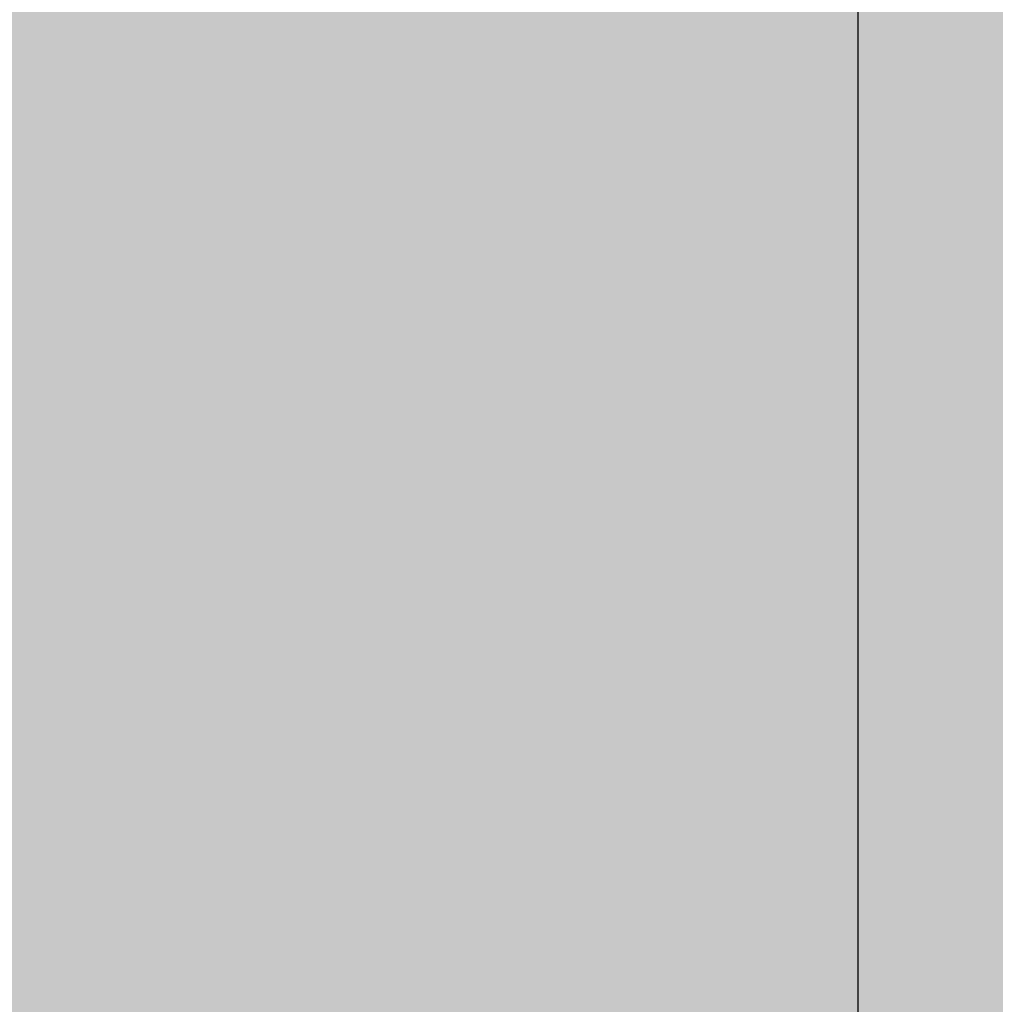
# Model space of a CAD drawing. Units: millimetres. Extents: x -22994 to 29398, y -19990 to 20176.
# Tile 50 of 135: x 183.63 to 197.67, y 110.33 to 124.5. Entities that reach past the tile are written whole.
import ezdxf

# ---------------------------------------------------------------- set-up
doc = ezdxf.new("R2010")
doc.units = ezdxf.units.MM
doc.header["$MEASUREMENT"] = 0
for name, color, linetype, lineweight in [('M-DIMS', 2, 'Continuous', 18), ('M-EQPM', 7, 'Continuous', 25), ('M-EQPM-PATT', 7, 'Continuous', 18)]:
    doc.layers.add(name, color=color, linetype=linetype, lineweight=lineweight)
doc.styles.get("Standard").update_dxf_attribs({"font": 'arial.ttf'})
doc.dimstyles.get("Standard").update_dxf_attribs({"dimtxt": 0.18, "dimasz": 10000, "dimexe": 0.18, "dimexo": 0.0625, "dimgap": 0.09, "dimtad": 0, "dimtih": 1, "dimtoh": 1, "dimdec": 0, "dimzin": 0, "dimdsep": 46, "dimtxsty": 'Standard', "dimcen": 0.09, "dimadec": 0, "dimazin": 0, "dimtfac": 1, "dimtdec": 0, "dimtofl": 0, "dimtmove": 0, "dimatfit": 3, "dimfxl": 1, "dimtolj": 1, "dimtzin": 0, "dimlwd": 30, "dimarcsym": 0})

# ---------------------------------------------------------------- blocks, each defined once
blk = doc.blocks.new('*D2')
at = {"layer": 'Defpoints', "color": 0, "transparency": 16777216}
for p in [(6.677, 10.271), (290.852, 10.271), (290.852, -5.079)]:
    blk.add_point(p, dxfattribs=at)
at = {"layer": 'M-DIMS', "color": 0, "lineweight": -2, "transparency": 16777216}
for p, q in [((6.677, 10.209), (6.677, -5.259)), ((290.852, 10.209), (290.852, -5.259))]:
    blk.add_line(p, q, dxfattribs=at)
at = {"layer": 'M-DIMS', "color": 0, "lineweight": 30, "transparency": 16777216}
for p, q in [((-9993.323, -5.079), (-19993.323, -5.079)), ((10290.852, -5.079), (20290.852, -5.079))]:
    blk.add_line(p, q, dxfattribs=at)
at = {"layer": 'M-DIMS', "color": 0, "transparency": 16777216}
for points in [[(-9993.323, 1661.588), (-9993.323, -1671.745), (6.677, -5.079)], [(10290.852, 1661.588), (10290.852, -1671.745), (290.852, -5.079)]]:
    blk.add_solid(points, dxfattribs=at)
at = {"layer": 'M-DIMS', "color": 0, "transparency": 16777216, "insert": (148.765, -5.079), "char_height": 0.18, "attachment_point": 5}
blk.add_mtext('\\A1;284.2', dxfattribs=at)
blk = doc.blocks.new('*D3')
at = {"layer": 'Defpoints', "color": 0, "transparency": 16777216}
for p in [(110.265, 204.165), (110.265, 176.366), (95.833, 127.967)]:
    blk.add_point(p, dxfattribs=at)
at = {"layer": 'M-DIMS', "color": 0, "lineweight": -2, "transparency": 16777216}
for p, q in [((95.833, 128.03), (95.833, 204.345)), ((110.265, 176.429), (110.265, 204.345))]:
    blk.add_line(p, q, dxfattribs=at)
at = {"layer": 'M-DIMS', "color": 0, "lineweight": 30, "transparency": 16777216}
for p, q in [((-9904.167, 204.165), (-19904.167, 204.165)), ((10110.265, 204.165), (20110.265, 204.165))]:
    blk.add_line(p, q, dxfattribs=at)
at = {"layer": 'M-DIMS', "color": 0, "transparency": 16777216}
for points in [[(-9904.167, 1870.832), (-9904.167, -1462.501), (95.833, 204.165)], [(10110.265, 1870.832), (10110.265, -1462.501), (110.265, 204.165)]]:
    blk.add_solid(points, dxfattribs=at)
at = {"layer": 'M-DIMS', "color": 0, "transparency": 16777216, "insert": (103.049, 204.165), "char_height": 0.18, "attachment_point": 5}
blk.add_mtext('\\A1;14.432', dxfattribs=at)
blk = doc.blocks.new('*D4')
at = {"layer": 'Defpoints', "color": 0, "transparency": 16777216}
for p in [(116.265, 204.165), (110.265, 176.366), (116.265, 176.366)]:
    blk.add_point(p, dxfattribs=at)
at = {"layer": 'M-DIMS', "color": 0, "lineweight": -2, "transparency": 16777216}
for p, q in [((110.265, 176.429), (110.265, 204.345)), ((116.265, 176.429), (116.265, 204.345))]:
    blk.add_line(p, q, dxfattribs=at)
at = {"layer": 'M-DIMS', "color": 0, "lineweight": 30, "transparency": 16777216}
for p, q in [((-9889.735, 204.165), (-19889.735, 204.165)), ((10116.265, 204.165), (20116.265, 204.165))]:
    blk.add_line(p, q, dxfattribs=at)
at = {"layer": 'M-DIMS', "color": 0, "transparency": 16777216}
for points in [[(-9889.735, 1870.832), (-9889.735, -1462.501), (110.265, 204.165)], [(10116.265, 1870.832), (10116.265, -1462.501), (116.265, 204.165)]]:
    blk.add_solid(points, dxfattribs=at)
at = {"layer": 'M-DIMS', "color": 0, "transparency": 16777216, "insert": (113.265, 204.165), "char_height": 0.18, "attachment_point": 5}
blk.add_mtext('\\A1;6', dxfattribs=at)
blk = doc.blocks.new('*D5')
at = {"layer": 'Defpoints', "color": 0, "transparency": 16777216}
for p in [(181.265, 204.165), (116.265, 176.366), (181.265, 176.366)]:
    blk.add_point(p, dxfattribs=at)
at = {"layer": 'M-DIMS', "color": 0, "lineweight": -2, "transparency": 16777216}
for p, q in [((116.265, 176.429), (116.265, 204.345)), ((181.265, 176.429), (181.265, 204.345))]:
    blk.add_line(p, q, dxfattribs=at)
at = {"layer": 'M-DIMS', "color": 0, "lineweight": 30, "transparency": 16777216}
for p, q in [((-9883.735, 204.165), (-19883.735, 204.165)), ((10181.265, 204.165), (20181.265, 204.165))]:
    blk.add_line(p, q, dxfattribs=at)
at = {"layer": 'M-DIMS', "color": 0, "transparency": 16777216}
for points in [[(-9883.735, 1870.832), (-9883.735, -1462.501), (116.265, 204.165)], [(10181.265, 1870.832), (10181.265, -1462.501), (181.265, 204.165)]]:
    blk.add_solid(points, dxfattribs=at)
at = {"layer": 'M-DIMS', "color": 0, "transparency": 16777216, "insert": (148.765, 204.165), "char_height": 0.18, "attachment_point": 5}
blk.add_mtext('\\A1;65', dxfattribs=at)
blk = doc.blocks.new('*D6')
at = {"layer": 'Defpoints', "color": 0, "transparency": 16777216}
for p in [(187.265, 204.165), (181.265, 176.366), (187.265, 176.366)]:
    blk.add_point(p, dxfattribs=at)
at = {"layer": 'M-DIMS', "color": 0, "lineweight": -2, "transparency": 16777216}
for p, q in [((181.265, 176.429), (181.265, 204.345)), ((187.265, 176.429), (187.265, 204.345))]:
    blk.add_line(p, q, dxfattribs=at)
at = {"layer": 'M-DIMS', "color": 0, "lineweight": 30, "transparency": 16777216}
for p, q in [((-9818.735, 204.165), (-19818.735, 204.165)), ((10187.265, 204.165), (20187.265, 204.165))]:
    blk.add_line(p, q, dxfattribs=at)
at = {"layer": 'M-DIMS', "color": 0, "transparency": 16777216}
for points in [[(-9818.735, 1870.832), (-9818.735, -1462.501), (181.265, 204.165)], [(10187.265, 1870.832), (10187.265, -1462.501), (187.265, 204.165)]]:
    blk.add_solid(points, dxfattribs=at)
at = {"layer": 'M-DIMS', "color": 0, "transparency": 16777216, "insert": (184.265, 204.165), "char_height": 0.18, "attachment_point": 5}
blk.add_mtext('\\A1;6', dxfattribs=at)
blk = doc.blocks.new('*D7')
at = {"layer": 'Defpoints', "color": 0, "transparency": 16777216}
for p in [(201.697, 204.165), (187.265, 176.366), (201.697, 127.967)]:
    blk.add_point(p, dxfattribs=at)
at = {"layer": 'M-DIMS', "color": 0, "lineweight": -2, "transparency": 16777216}
for p, q in [((187.265, 176.429), (187.265, 204.345)), ((201.697, 128.03), (201.697, 204.345))]:
    blk.add_line(p, q, dxfattribs=at)
at = {"layer": 'M-DIMS', "color": 0, "lineweight": 30, "transparency": 16777216}
for p, q in [((-9812.735, 204.165), (-19812.735, 204.165)), ((10201.697, 204.165), (20201.697, 204.165))]:
    blk.add_line(p, q, dxfattribs=at)
at = {"layer": 'M-DIMS', "color": 0, "transparency": 16777216}
for points in [[(-9812.735, 1870.832), (-9812.735, -1462.501), (187.265, 204.165)], [(10201.697, 1870.832), (10201.697, -1462.501), (201.697, 204.165)]]:
    blk.add_solid(points, dxfattribs=at)
at = {"layer": 'M-DIMS', "color": 0, "transparency": 16777216, "insert": (194.481, 204.165), "char_height": 0.18, "attachment_point": 5}
blk.add_mtext('\\A1;14.432', dxfattribs=at)
blk = doc.blocks.new('*D8')
at = {"layer": 'Defpoints', "color": 0, "transparency": 16777216}
for p in [(227.648, 204.165), (227.648, 146.73), (201.697, 127.967)]:
    blk.add_point(p, dxfattribs=at)
at = {"layer": 'M-DIMS', "color": 0, "lineweight": -2, "transparency": 16777216}
for p, q in [((201.697, 128.03), (201.697, 204.345)), ((227.648, 146.792), (227.648, 204.345))]:
    blk.add_line(p, q, dxfattribs=at)
at = {"layer": 'M-DIMS', "color": 0, "lineweight": 30, "transparency": 16777216}
for p, q in [((-9798.303, 204.165), (-19798.303, 204.165)), ((10227.648, 204.165), (20227.648, 204.165))]:
    blk.add_line(p, q, dxfattribs=at)
at = {"layer": 'M-DIMS', "color": 0, "transparency": 16777216}
for points in [[(-9798.303, 1870.832), (-9798.303, -1462.501), (201.697, 204.165)], [(10227.648, 1870.832), (10227.648, -1462.501), (227.648, 204.165)]]:
    blk.add_solid(points, dxfattribs=at)
at = {"layer": 'M-DIMS', "color": 0, "transparency": 16777216, "insert": (214.673, 204.165), "char_height": 0.18, "attachment_point": 5}
blk.add_mtext('\\A1;25.95', dxfattribs=at)
blk = doc.blocks.new('*D9')
at = {"layer": 'Defpoints', "color": 0, "transparency": 16777216}
for p in [(187.265, 176.366), (306.202, 176.366), (290.852, 10.271)]:
    blk.add_point(p, dxfattribs=at)
at = {"layer": 'M-DIMS', "color": 0, "lineweight": 30, "transparency": 16777216}
for p, q in [((306.202, 10176.366), (306.202, 20176.366)), ((306.202, -9989.729), (306.202, -19989.729))]:
    blk.add_line(p, q, dxfattribs=at)
at = {"layer": 'M-DIMS', "color": 0, "lineweight": -2, "transparency": 16777216}
for p, q in [((187.327, 176.366), (306.382, 176.366)), ((290.915, 10.271), (306.382, 10.271))]:
    blk.add_line(p, q, dxfattribs=at)
at = {"layer": 'M-DIMS', "color": 0, "transparency": 16777216}
for points in [[(-1360.465, 10176.366), (1972.869, 10176.366), (306.202, 176.366)], [(-1360.465, -9989.729), (1972.869, -9989.729), (306.202, 10.271)]]:
    blk.add_solid(points, dxfattribs=at)
at = {"layer": 'M-DIMS', "color": 0, "transparency": 16777216, "insert": (306.202, 93.319), "char_height": 0.18, "attachment_point": 5}
blk.add_mtext('\\A1;166.1', dxfattribs=at)
blk = doc.blocks.new('*D10')
at = {"layer": 'Defpoints', "color": 0, "transparency": 16777216}
for p in [(125.65, 136.071), (133.346, 136.071), (133.346, -5.079)]:
    blk.add_point(p, dxfattribs=at)
at = {"layer": 'M-DIMS', "color": 0, "lineweight": -2, "transparency": 16777216}
for p, q in [((125.65, 136.009), (125.65, -5.259)), ((133.346, 136.009), (133.346, -5.259))]:
    blk.add_line(p, q, dxfattribs=at)
at = {"layer": 'M-DIMS', "color": 0, "lineweight": 30, "transparency": 16777216}
for p, q in [((-9874.35, -5.079), (-19874.35, -5.079)), ((10133.346, -5.079), (20133.346, -5.079))]:
    blk.add_line(p, q, dxfattribs=at)
at = {"layer": 'M-DIMS', "color": 0, "transparency": 16777216}
for points in [[(-9874.35, 1661.588), (-9874.35, -1671.745), (125.65, -5.079)], [(10133.346, 1661.588), (10133.346, -1671.745), (133.346, -5.079)]]:
    blk.add_solid(points, dxfattribs=at)
at = {"layer": 'M-DIMS', "color": 0, "transparency": 16777216, "insert": (129.498, -5.079), "char_height": 0.18, "attachment_point": 5}
blk.add_mtext('\\A1;7.696', dxfattribs=at)
blk = doc.blocks.new('*D11')
at = {"layer": 'Defpoints', "color": 0, "transparency": 16777216}
for p in [(133.346, 136.071), (135.65, 136.071), (135.65, -5.079)]:
    blk.add_point(p, dxfattribs=at)
at = {"layer": 'M-DIMS', "color": 0, "lineweight": -2, "transparency": 16777216}
for p, q in [((133.346, 136.009), (133.346, -5.259)), ((135.65, 136.009), (135.65, -5.259))]:
    blk.add_line(p, q, dxfattribs=at)
at = {"layer": 'M-DIMS', "color": 0, "lineweight": 30, "transparency": 16777216}
for p, q in [((-9866.654, -5.079), (-19866.654, -5.079)), ((10135.65, -5.079), (20135.65, -5.079))]:
    blk.add_line(p, q, dxfattribs=at)
at = {"layer": 'M-DIMS', "color": 0, "transparency": 16777216}
for points in [[(-9866.654, 1661.588), (-9866.654, -1671.745), (133.346, -5.079)], [(10135.65, 1661.588), (10135.65, -1671.745), (135.65, -5.079)]]:
    blk.add_solid(points, dxfattribs=at)
at = {"layer": 'M-DIMS', "color": 0, "transparency": 16777216, "insert": (134.498, -5.079), "char_height": 0.18, "attachment_point": 5}
blk.add_mtext('\\A1;2.304', dxfattribs=at)
blk = doc.blocks.new('*D12')
at = {"layer": 'Defpoints', "color": 0, "transparency": 16777216}
for p in [(135.65, 136.071), (145.65, 136.071), (145.65, -5.079)]:
    blk.add_point(p, dxfattribs=at)
at = {"layer": 'M-DIMS', "color": 0, "lineweight": -2, "transparency": 16777216}
for p, q in [((135.65, 136.009), (135.65, -5.259)), ((145.65, 136.009), (145.65, -5.259))]:
    blk.add_line(p, q, dxfattribs=at)
at = {"layer": 'M-DIMS', "color": 0, "lineweight": 30, "transparency": 16777216}
for p, q in [((-9864.35, -5.079), (-19864.35, -5.079)), ((10145.65, -5.079), (20145.65, -5.079))]:
    blk.add_line(p, q, dxfattribs=at)
at = {"layer": 'M-DIMS', "color": 0, "transparency": 16777216}
for points in [[(-9864.35, 1661.588), (-9864.35, -1671.745), (135.65, -5.079)], [(10145.65, 1661.588), (10145.65, -1671.745), (145.65, -5.079)]]:
    blk.add_solid(points, dxfattribs=at)
at = {"layer": 'M-DIMS', "color": 0, "transparency": 16777216, "insert": (140.65, -5.079), "char_height": 0.18, "attachment_point": 5}
blk.add_mtext('\\A1;10', dxfattribs=at)
blk = doc.blocks.new('*D13')
at = {"layer": 'Defpoints', "color": 0, "transparency": 16777216}
for p in [(145.65, 136.071), (155.65, 136.071), (155.65, -5.079)]:
    blk.add_point(p, dxfattribs=at)
at = {"layer": 'M-DIMS', "color": 0, "lineweight": -2, "transparency": 16777216}
for p, q in [((145.65, 136.009), (145.65, -5.259)), ((155.65, 136.009), (155.65, -5.259))]:
    blk.add_line(p, q, dxfattribs=at)
at = {"layer": 'M-DIMS', "color": 0, "lineweight": 30, "transparency": 16777216}
for p, q in [((-9854.35, -5.079), (-19854.35, -5.079)), ((10155.65, -5.079), (20155.65, -5.079))]:
    blk.add_line(p, q, dxfattribs=at)
at = {"layer": 'M-DIMS', "color": 0, "transparency": 16777216}
for points in [[(-9854.35, 1661.588), (-9854.35, -1671.745), (145.65, -5.079)], [(10155.65, 1661.588), (10155.65, -1671.745), (155.65, -5.079)]]:
    blk.add_solid(points, dxfattribs=at)
at = {"layer": 'M-DIMS', "color": 0, "transparency": 16777216, "insert": (150.65, -5.079), "char_height": 0.18, "attachment_point": 5}
blk.add_mtext('\\A1;10', dxfattribs=at)
blk = doc.blocks.new('*D14')
at = {"layer": 'Defpoints', "color": 0, "transparency": 16777216}
for p in [(155.65, 136.071), (165.65, 136.071), (165.65, -5.079)]:
    blk.add_point(p, dxfattribs=at)
at = {"layer": 'M-DIMS', "color": 0, "lineweight": -2, "transparency": 16777216}
for p, q in [((155.65, 136.009), (155.65, -5.259)), ((165.65, 136.009), (165.65, -5.259))]:
    blk.add_line(p, q, dxfattribs=at)
at = {"layer": 'M-DIMS', "color": 0, "lineweight": 30, "transparency": 16777216}
for p, q in [((-9844.35, -5.079), (-19844.35, -5.079)), ((10165.65, -5.079), (20165.65, -5.079))]:
    blk.add_line(p, q, dxfattribs=at)
at = {"layer": 'M-DIMS', "color": 0, "transparency": 16777216}
for points in [[(-9844.35, 1661.588), (-9844.35, -1671.745), (155.65, -5.079)], [(10165.65, 1661.588), (10165.65, -1671.745), (165.65, -5.079)]]:
    blk.add_solid(points, dxfattribs=at)
at = {"layer": 'M-DIMS', "color": 0, "transparency": 16777216, "insert": (160.65, -5.079), "char_height": 0.18, "attachment_point": 5}
blk.add_mtext('\\A1;10', dxfattribs=at)
blk = doc.blocks.new('*D15')
at = {"layer": 'Defpoints', "color": 0, "transparency": 16777216}
for p in [(173.346, 154.788), (173.346, 136.071), (306.202, 136.071)]:
    blk.add_point(p, dxfattribs=at)
at = {"layer": 'M-DIMS', "color": 0, "lineweight": 30, "transparency": 16777216}
for p, q in [((306.202, 10154.788), (306.202, 20154.788)), ((306.202, -9863.929), (306.202, -19863.929))]:
    blk.add_line(p, q, dxfattribs=at)
at = {"layer": 'M-DIMS', "color": 0, "lineweight": -2, "transparency": 16777216}
for p, q in [((173.408, 154.788), (306.382, 154.788)), ((173.408, 136.071), (306.382, 136.071))]:
    blk.add_line(p, q, dxfattribs=at)
at = {"layer": 'M-DIMS', "color": 0, "transparency": 16777216}
for points in [[(-1360.465, 10154.788), (1972.869, 10154.788), (306.202, 154.788)], [(-1360.465, -9863.929), (1972.869, -9863.929), (306.202, 136.071)]]:
    blk.add_solid(points, dxfattribs=at)
at = {"layer": 'M-DIMS', "color": 0, "transparency": 16777216, "insert": (306.202, 145.43), "char_height": 0.18, "attachment_point": 5}
blk.add_mtext('\\A1;18.717', dxfattribs=at)
blk = doc.blocks.new('*D16')
at = {"layer": 'Defpoints', "color": 0, "transparency": 16777216}
for p in [(120.17, 204.165), (110.466, 48.035), (120.17, 48.035)]:
    blk.add_point(p, dxfattribs=at)
at = {"layer": 'M-DIMS', "color": 0, "lineweight": -2, "transparency": 16777216}
for p, q in [((110.466, 48.097), (110.466, 204.345)), ((120.17, 48.097), (120.17, 204.345))]:
    blk.add_line(p, q, dxfattribs=at)
at = {"layer": 'M-DIMS', "color": 0, "lineweight": 30, "transparency": 16777216}
for p, q in [((-9889.534, 204.165), (-19889.534, 204.165)), ((10120.17, 204.165), (20120.17, 204.165))]:
    blk.add_line(p, q, dxfattribs=at)
at = {"layer": 'M-DIMS', "color": 0, "transparency": 16777216}
for points in [[(-9889.534, 1870.832), (-9889.534, -1462.501), (110.466, 204.165)], [(10120.17, 1870.832), (10120.17, -1462.501), (120.17, 204.165)]]:
    blk.add_solid(points, dxfattribs=at)
at = {"layer": 'M-DIMS', "color": 0, "transparency": 16777216, "insert": (115.318, 204.165), "char_height": 0.18, "attachment_point": 5}
blk.add_mtext('\\A1;9.704', dxfattribs=at)
blk = doc.blocks.new('*D17')
at = {"layer": 'Defpoints', "color": 0, "transparency": 16777216}
for p in [(126.17, 204.165), (120.17, 48.035), (126.17, 48.035)]:
    blk.add_point(p, dxfattribs=at)
at = {"layer": 'M-DIMS', "color": 0, "lineweight": -2, "transparency": 16777216}
for p, q in [((120.17, 48.097), (120.17, 204.345)), ((126.17, 48.097), (126.17, 204.345))]:
    blk.add_line(p, q, dxfattribs=at)
at = {"layer": 'M-DIMS', "color": 0, "lineweight": 30, "transparency": 16777216}
for p, q in [((-9879.83, 204.165), (-19879.83, 204.165)), ((10126.17, 204.165), (20126.17, 204.165))]:
    blk.add_line(p, q, dxfattribs=at)
at = {"layer": 'M-DIMS', "color": 0, "transparency": 16777216}
for points in [[(-9879.83, 1870.832), (-9879.83, -1462.501), (120.17, 204.165)], [(10126.17, 1870.832), (10126.17, -1462.501), (126.17, 204.165)]]:
    blk.add_solid(points, dxfattribs=at)
at = {"layer": 'M-DIMS', "color": 0, "transparency": 16777216, "insert": (123.17, 204.165), "char_height": 0.18, "attachment_point": 5}
blk.add_mtext('\\A1;6', dxfattribs=at)
blk = doc.blocks.new('*D18')
at = {"layer": 'Defpoints', "color": 0, "transparency": 16777216}
for p in [(132.17, 204.165), (126.17, 48.035), (132.17, 48.035)]:
    blk.add_point(p, dxfattribs=at)
at = {"layer": 'M-DIMS', "color": 0, "lineweight": -2, "transparency": 16777216}
for p, q in [((126.17, 48.097), (126.17, 204.345)), ((132.17, 48.097), (132.17, 204.345))]:
    blk.add_line(p, q, dxfattribs=at)
at = {"layer": 'M-DIMS', "color": 0, "lineweight": 30, "transparency": 16777216}
for p, q in [((-9873.83, 204.165), (-19873.83, 204.165)), ((10132.17, 204.165), (20132.17, 204.165))]:
    blk.add_line(p, q, dxfattribs=at)
at = {"layer": 'M-DIMS', "color": 0, "transparency": 16777216}
for points in [[(-9873.83, 1870.832), (-9873.83, -1462.501), (126.17, 204.165)], [(10132.17, 1870.832), (10132.17, -1462.501), (132.17, 204.165)]]:
    blk.add_solid(points, dxfattribs=at)
at = {"layer": 'M-DIMS', "color": 0, "transparency": 16777216, "insert": (129.17, 204.165), "char_height": 0.18, "attachment_point": 5}
blk.add_mtext('\\A1;6', dxfattribs=at)
blk = doc.blocks.new('*D19')
at = {"layer": 'Defpoints', "color": 0, "transparency": 16777216}
for p in [(138.17, 204.165), (132.17, 48.035), (138.17, 48.035)]:
    blk.add_point(p, dxfattribs=at)
at = {"layer": 'M-DIMS', "color": 0, "lineweight": -2, "transparency": 16777216}
for p, q in [((132.17, 48.097), (132.17, 204.345)), ((138.17, 48.097), (138.17, 204.345))]:
    blk.add_line(p, q, dxfattribs=at)
at = {"layer": 'M-DIMS', "color": 0, "lineweight": 30, "transparency": 16777216}
for p, q in [((-9867.83, 204.165), (-19867.83, 204.165)), ((10138.17, 204.165), (20138.17, 204.165))]:
    blk.add_line(p, q, dxfattribs=at)
at = {"layer": 'M-DIMS', "color": 0, "transparency": 16777216}
for points in [[(-9867.83, 1870.832), (-9867.83, -1462.501), (132.17, 204.165)], [(10138.17, 1870.832), (10138.17, -1462.501), (138.17, 204.165)]]:
    blk.add_solid(points, dxfattribs=at)
at = {"layer": 'M-DIMS', "color": 0, "transparency": 16777216, "insert": (135.17, 204.165), "char_height": 0.18, "attachment_point": 5}
blk.add_mtext('\\A1;6', dxfattribs=at)
blk = doc.blocks.new('*D20')
at = {"layer": 'Defpoints', "color": 0, "transparency": 16777216}
for p in [(144.17, 204.165), (138.17, 48.035), (144.17, 48.035)]:
    blk.add_point(p, dxfattribs=at)
at = {"layer": 'M-DIMS', "color": 0, "lineweight": -2, "transparency": 16777216}
for p, q in [((138.17, 48.097), (138.17, 204.345)), ((144.17, 48.097), (144.17, 204.345))]:
    blk.add_line(p, q, dxfattribs=at)
at = {"layer": 'M-DIMS', "color": 0, "lineweight": 30, "transparency": 16777216}
for p, q in [((-9861.83, 204.165), (-19861.83, 204.165)), ((10144.17, 204.165), (20144.17, 204.165))]:
    blk.add_line(p, q, dxfattribs=at)
at = {"layer": 'M-DIMS', "color": 0, "transparency": 16777216}
for points in [[(-9861.83, 1870.832), (-9861.83, -1462.501), (138.17, 204.165)], [(10144.17, 1870.832), (10144.17, -1462.501), (144.17, 204.165)]]:
    blk.add_solid(points, dxfattribs=at)
at = {"layer": 'M-DIMS', "color": 0, "transparency": 16777216, "insert": (141.17, 204.165), "char_height": 0.18, "attachment_point": 5}
blk.add_mtext('\\A1;6', dxfattribs=at)
blk = doc.blocks.new('*D21')
at = {"layer": 'Defpoints', "color": 0, "transparency": 16777216}
for p in [(149.116, 204.165), (144.17, 48.035), (149.116, 48.035)]:
    blk.add_point(p, dxfattribs=at)
at = {"layer": 'M-DIMS', "color": 0, "lineweight": -2, "transparency": 16777216}
for p, q in [((144.17, 48.097), (144.17, 204.345)), ((149.116, 48.097), (149.116, 204.345))]:
    blk.add_line(p, q, dxfattribs=at)
at = {"layer": 'M-DIMS', "color": 0, "lineweight": 30, "transparency": 16777216}
for p, q in [((-9855.83, 204.165), (-19855.83, 204.165)), ((10149.116, 204.165), (20149.116, 204.165))]:
    blk.add_line(p, q, dxfattribs=at)
at = {"layer": 'M-DIMS', "color": 0, "transparency": 16777216}
for points in [[(-9855.83, 1870.832), (-9855.83, -1462.501), (144.17, 204.165)], [(10149.116, 1870.832), (10149.116, -1462.501), (149.116, 204.165)]]:
    blk.add_solid(points, dxfattribs=at)
at = {"layer": 'M-DIMS', "color": 0, "transparency": 16777216, "insert": (146.643, 204.165), "char_height": 0.18, "attachment_point": 5}
blk.add_mtext('\\A1;4.945', dxfattribs=at)
blk = doc.blocks.new('*D22')
at = {"layer": 'Defpoints', "color": 0, "transparency": 16777216}
for p in [(149.116, 30.99), (155.116, 30.99), (155.116, -5.079)]:
    blk.add_point(p, dxfattribs=at)
at = {"layer": 'M-DIMS', "color": 0, "lineweight": -2, "transparency": 16777216}
for p, q in [((149.116, 30.927), (149.116, -5.259)), ((155.116, 30.927), (155.116, -5.259))]:
    blk.add_line(p, q, dxfattribs=at)
at = {"layer": 'M-DIMS', "color": 0, "lineweight": 30, "transparency": 16777216}
for p, q in [((-9850.884, -5.079), (-19850.884, -5.079)), ((10155.116, -5.079), (20155.116, -5.079))]:
    blk.add_line(p, q, dxfattribs=at)
at = {"layer": 'M-DIMS', "color": 0, "transparency": 16777216}
for points in [[(-9850.884, 1661.588), (-9850.884, -1671.745), (149.116, -5.079)], [(10155.116, 1661.588), (10155.116, -1671.745), (155.116, -5.079)]]:
    blk.add_solid(points, dxfattribs=at)
at = {"layer": 'M-DIMS', "color": 0, "transparency": 16777216, "insert": (152.116, -5.079), "char_height": 0.18, "attachment_point": 5}
blk.add_mtext('\\A1;6', dxfattribs=at)
blk = doc.blocks.new('*D23')
at = {"layer": 'Defpoints', "color": 0, "transparency": 16777216}
for p in [(155.116, 30.99), (161.116, 30.99), (161.116, -5.079)]:
    blk.add_point(p, dxfattribs=at)
at = {"layer": 'M-DIMS', "color": 0, "lineweight": -2, "transparency": 16777216}
for p, q in [((155.116, 30.927), (155.116, -5.259)), ((161.116, 30.927), (161.116, -5.259))]:
    blk.add_line(p, q, dxfattribs=at)
at = {"layer": 'M-DIMS', "color": 0, "lineweight": 30, "transparency": 16777216}
for p, q in [((-9844.884, -5.079), (-19844.884, -5.079)), ((10161.116, -5.079), (20161.116, -5.079))]:
    blk.add_line(p, q, dxfattribs=at)
at = {"layer": 'M-DIMS', "color": 0, "transparency": 16777216}
for points in [[(-9844.884, 1661.588), (-9844.884, -1671.745), (155.116, -5.079)], [(10161.116, 1661.588), (10161.116, -1671.745), (161.116, -5.079)]]:
    blk.add_solid(points, dxfattribs=at)
at = {"layer": 'M-DIMS', "color": 0, "transparency": 16777216, "insert": (158.116, -5.079), "char_height": 0.18, "attachment_point": 5}
blk.add_mtext('\\A1;6', dxfattribs=at)
blk = doc.blocks.new('*D24')
at = {"layer": 'Defpoints', "color": 0, "transparency": 16777216}
for p in [(161.116, 30.99), (166.439, 30.99), (166.439, -5.079)]:
    blk.add_point(p, dxfattribs=at)
at = {"layer": 'M-DIMS', "color": 0, "lineweight": -2, "transparency": 16777216}
for p, q in [((161.116, 30.927), (161.116, -5.259)), ((166.439, 30.927), (166.439, -5.259))]:
    blk.add_line(p, q, dxfattribs=at)
at = {"layer": 'M-DIMS', "color": 0, "lineweight": 30, "transparency": 16777216}
for p, q in [((-9838.884, -5.079), (-19838.884, -5.079)), ((10166.439, -5.079), (20166.439, -5.079))]:
    blk.add_line(p, q, dxfattribs=at)
at = {"layer": 'M-DIMS', "color": 0, "transparency": 16777216}
for points in [[(-9838.884, 1661.588), (-9838.884, -1671.745), (161.116, -5.079)], [(10166.439, 1661.588), (10166.439, -1671.745), (166.439, -5.079)]]:
    blk.add_solid(points, dxfattribs=at)
at = {"layer": 'M-DIMS', "color": 0, "transparency": 16777216, "insert": (163.777, -5.079), "char_height": 0.18, "attachment_point": 5}
blk.add_mtext('\\A1;5.323', dxfattribs=at)
blk = doc.blocks.new('*D25')
at = {"layer": 'Defpoints', "color": 0, "transparency": 16777216}
for p in [(166.439, 30.99), (172.439, 30.99), (172.439, -5.079)]:
    blk.add_point(p, dxfattribs=at)
at = {"layer": 'M-DIMS', "color": 0, "lineweight": -2, "transparency": 16777216}
for p, q in [((166.439, 30.927), (166.439, -5.259)), ((172.439, 30.927), (172.439, -5.259))]:
    blk.add_line(p, q, dxfattribs=at)
at = {"layer": 'M-DIMS', "color": 0, "lineweight": 30, "transparency": 16777216}
for p, q in [((-9833.561, -5.079), (-19833.561, -5.079)), ((10172.439, -5.079), (20172.439, -5.079))]:
    blk.add_line(p, q, dxfattribs=at)
at = {"layer": 'M-DIMS', "color": 0, "transparency": 16777216}
for points in [[(-9833.561, 1661.588), (-9833.561, -1671.745), (166.439, -5.079)], [(10172.439, 1661.588), (10172.439, -1671.745), (172.439, -5.079)]]:
    blk.add_solid(points, dxfattribs=at)
at = {"layer": 'M-DIMS', "color": 0, "transparency": 16777216, "insert": (169.439, -5.079), "char_height": 0.18, "attachment_point": 5}
blk.add_mtext('\\A1;6', dxfattribs=at)
blk = doc.blocks.new('*D26')
at = {"layer": 'Defpoints', "color": 0, "transparency": 16777216}
for p in [(172.439, 30.99), (178.439, 30.99), (178.439, -5.079)]:
    blk.add_point(p, dxfattribs=at)
at = {"layer": 'M-DIMS', "color": 0, "lineweight": -2, "transparency": 16777216}
for p, q in [((172.439, 30.927), (172.439, -5.259)), ((178.439, 30.927), (178.439, -5.259))]:
    blk.add_line(p, q, dxfattribs=at)
at = {"layer": 'M-DIMS', "color": 0, "lineweight": 30, "transparency": 16777216}
for p, q in [((-9827.561, -5.079), (-19827.561, -5.079)), ((10178.439, -5.079), (20178.439, -5.079))]:
    blk.add_line(p, q, dxfattribs=at)
at = {"layer": 'M-DIMS', "color": 0, "transparency": 16777216}
for points in [[(-9827.561, 1661.588), (-9827.561, -1671.745), (172.439, -5.079)], [(10178.439, 1661.588), (10178.439, -1671.745), (178.439, -5.079)]]:
    blk.add_solid(points, dxfattribs=at)
at = {"layer": 'M-DIMS', "color": 0, "transparency": 16777216, "insert": (175.439, -5.079), "char_height": 0.18, "attachment_point": 5}
blk.add_mtext('\\A1;6', dxfattribs=at)
blk = doc.blocks.new('*D27')
at = {"layer": 'Defpoints', "color": 0, "transparency": 16777216}
for p in [(178.439, 30.99), (188.117, 30.99), (188.117, -5.079)]:
    blk.add_point(p, dxfattribs=at)
at = {"layer": 'M-DIMS', "color": 0, "lineweight": -2, "transparency": 16777216}
for p, q in [((178.439, 30.927), (178.439, -5.259)), ((188.117, 30.927), (188.117, -5.259))]:
    blk.add_line(p, q, dxfattribs=at)
at = {"layer": 'M-DIMS', "color": 0, "lineweight": 30, "transparency": 16777216}
for p, q in [((-9821.561, -5.079), (-19821.561, -5.079)), ((10188.117, -5.079), (20188.117, -5.079))]:
    blk.add_line(p, q, dxfattribs=at)
at = {"layer": 'M-DIMS', "color": 0, "transparency": 16777216}
for points in [[(-9821.561, 1661.588), (-9821.561, -1671.745), (178.439, -5.079)], [(10188.117, 1661.588), (10188.117, -1671.745), (188.117, -5.079)]]:
    blk.add_solid(points, dxfattribs=at)
at = {"layer": 'M-DIMS', "color": 0, "transparency": 16777216, "insert": (183.278, -5.079), "char_height": 0.18, "attachment_point": 5}
blk.add_mtext('\\A1;9.679', dxfattribs=at)
blk = doc.blocks.new('*D28')
at = {"layer": 'Defpoints', "color": 0, "transparency": 16777216}
for p in [(188.117, 48.035), (306.202, 48.035), (188.117, 30.99)]:
    blk.add_point(p, dxfattribs=at)
at = {"layer": 'M-DIMS', "color": 0, "lineweight": 30, "transparency": 16777216}
for p, q in [((306.202, 10048.035), (306.202, 20048.035)), ((306.202, -9969.01), (306.202, -19969.01))]:
    blk.add_line(p, q, dxfattribs=at)
at = {"layer": 'M-DIMS', "color": 0, "lineweight": -2, "transparency": 16777216}
for p, q in [((188.18, 48.035), (306.382, 48.035)), ((188.18, 30.99), (306.382, 30.99))]:
    blk.add_line(p, q, dxfattribs=at)
at = {"layer": 'M-DIMS', "color": 0, "transparency": 16777216}
for points in [[(-1360.465, 10048.035), (1972.869, 10048.035), (306.202, 48.035)], [(-1360.465, -9969.01), (1972.869, -9969.01), (306.202, 30.99)]]:
    blk.add_solid(points, dxfattribs=at)
at = {"layer": 'M-DIMS', "color": 0, "transparency": 16777216, "insert": (306.202, 39.512), "char_height": 0.18, "attachment_point": 5}
blk.add_mtext('\\A1;17.045', dxfattribs=at)
blk = doc.blocks.new('*D29')
at = {"layer": 'Defpoints', "color": 0, "transparency": 16777216}
for p in [(36.801, 80.045), (64.03, 80.045)]:
    blk.add_point(p, dxfattribs=at)
at = {"layer": 'M-DIMS', "color": 0, "lineweight": -2, "transparency": 16777216}
for p, q in [((50.325, 80.045), (50.505, 80.045)), ((50.415, 79.955), (50.415, 80.135))]:
    blk.add_line(p, q, dxfattribs=at)
at = {"layer": 'M-DIMS', "color": 0, "lineweight": 30, "transparency": 16777216}
blk.add_line((20064.03, 80.03), (10064.03, 80.038), dxfattribs=at)
at = {"layer": 'M-DIMS', "color": 0, "transparency": 16777216}
blk.add_solid([(10064.031, 1746.704), (10064.028, -1586.629), (64.03, 80.045)], dxfattribs=at)
at = {"layer": 'M-DIMS', "color": 0, "transparency": 16777216, "insert": (20064.521, 80.03), "char_height": 0.18, "attachment_point": 5}
blk.add_mtext('\\A1;∅27.23', dxfattribs=at)
blk = doc.blocks.new('*D34')
at = {"layer": 'Defpoints', "color": 0, "transparency": 16777216}
for p in [(178.58, 122.895), (176.812, 121.128)]:
    blk.add_point(p, dxfattribs=at)
at = {"layer": 'M-DIMS', "color": 0, "lineweight": 30, "transparency": 16777216}
for p, q in [((14322.436, 14263.311), (7250.508, 7193.103)), ((24322.436, 14263.311), (14322.436, 14263.311))]:
    blk.add_line(p, q, dxfattribs=at)
at = {"layer": 'M-DIMS', "color": 0, "lineweight": -2, "transparency": 16777216}
for p, q in [((176.722, 121.128), (176.902, 121.128)), ((176.812, 121.038), (176.812, 121.218))]:
    blk.add_line(p, q, dxfattribs=at)
at = {"layer": 'M-DIMS', "color": 0, "transparency": 16777216}
blk.add_solid([(6072.14, 8371.758), (8428.876, 6014.448), (178.58, 122.895)], dxfattribs=at)
at = {"layer": 'M-DIMS', "color": 0, "transparency": 16777216, "insert": (24322.97, 14263.311), "char_height": 0.18, "attachment_point": 5}
blk.add_mtext('\\A1;6X R2.5', dxfattribs=at)
blk = doc.blocks.new('*D36')
at = {"layer": 'Defpoints', "color": 0, "transparency": 16777216}
for p in [(46.39, 31.303), (46.387, 26.593)]:
    blk.add_point(p, dxfattribs=at)
at = {"layer": 'M-DIMS', "color": 0, "lineweight": 30, "transparency": 16777216}
for p, q in [((57.15, 20031.301), (51.77, 10031.302)), ((10057.15, 20031.301), (57.15, 20031.301))]:
    blk.add_line(p, q, dxfattribs=at)
at = {"layer": 'M-DIMS', "color": 0, "lineweight": -2, "transparency": 16777216}
for p, q in [((46.299, 28.948), (46.479, 28.948)), ((46.389, 28.858), (46.389, 29.038))]:
    blk.add_line(p, q, dxfattribs=at)
at = {"layer": 'M-DIMS', "color": 0, "transparency": 16777216}
blk.add_solid([(-1614.896, 10032.199), (1718.436, 10030.405), (46.39, 31.303)], dxfattribs=at)
at = {"layer": 'M-DIMS', "color": 0, "transparency": 16777216, "insert": (10057.554, 20031.301), "char_height": 0.18, "attachment_point": 5}
blk.add_mtext('\\A1;∅4.71', dxfattribs=at)
blk = doc.blocks.new('*D37')
at = {"layer": 'Defpoints', "color": 0, "transparency": 16777216}
for p in [(54.834, 118.615), (59.494, 118.614)]:
    blk.add_point(p, dxfattribs=at)
at = {"layer": 'M-DIMS', "color": 0, "lineweight": -2, "transparency": 16777216}
for p, q in [((57.074, 118.614), (57.254, 118.614)), ((57.164, 118.524), (57.164, 118.704))]:
    blk.add_line(p, q, dxfattribs=at)
at = {"layer": 'M-DIMS', "color": 0, "lineweight": 30, "transparency": 16777216}
blk.add_line((20059.493, 116.253), (10059.494, 117.434), dxfattribs=at)
at = {"layer": 'M-DIMS', "color": 0, "transparency": 16777216}
blk.add_solid([(10059.69, 1784.1), (10059.297, -1549.233), (59.494, 118.614)], dxfattribs=at)
at = {"layer": 'M-DIMS', "color": 0, "transparency": 16777216, "insert": (20059.985, 116.253), "char_height": 0.18, "attachment_point": 5}
blk.add_mtext('\\A1;∅4.659', dxfattribs=at)

msp = doc.modelspace()

# ---------------------------------------------------------------- hatches: boundary and pattern name
at = {"layer": 'M-EQPM-PATT'}
h = msp.add_hatch(color=256, dxfattribs=at)
h.set_gradient(color1=(205, 32, 39), color2=(205, 32, 39), tint=1)
h.paths.add_polyline_path([(116.2647, 150.3662), (116.2647, 170.3662), (116.2647, 176.3662), (110.2647, 176.3662), (110.2647, 152.0276), (95.8327, 127.967), (95.8327, 16.6063), (201.6967, 16.6063), (201.6967, 127.967), (187.2647, 152.0276), (187.2647, 176.3662), (181.2647, 176.3662), (181.2647, 170.3662), (181.2647, 150.3662), (195.6967, 126.3055), (195.6967, 22.6063), (101.8327, 22.6063), (101.8327, 126.3055)])
h.paths.add_polyline_path([(185.2208, 88.6347), (101.8327, 88.6347), (101.8327, 87.6347), (182.8066, 87.6347), (178.7313, 83.5594), (195.6967, 83.5594), (195.6967, 84.5594), (181.1455, 84.5594)], flags=17)
h.paths.add_polyline_path([(95.8327, 88.6347), (60.9779, 88.6347, -0.0228552), (61.7178, 87.6347), (95.8327, 87.6347)])
h.paths.add_polyline_path([(215.6212, 86.5189), (215.6212, 80.5999), (220.5095, 83.5594)])
h.paths.add_polyline_path([(215.6212, 84.5594), (201.6967, 84.5594), (201.6967, 83.5594), (215.6212, 83.5594)])
h.paths.add_polyline_path([(225.3978, 86.5189), (220.5095, 83.5594), (225.3978, 80.5999)])
h.paths.add_polyline_path([(231.6256, 84.5594), (225.3978, 84.5594), (225.3978, 83.5594), (231.6256, 83.5594)])

# ---------------------------------------------------------------- linework, layer by layer
at = {"layer": 'M-EQPM'}
msp.add_lwpolyline([(116.2647, 170.3662), (116.2647, 150.3662), (101.8327, 126.3055), (101.8327, 22.6063), (195.6967, 22.6063), (195.6967, 126.3055), (181.2647, 150.3662), (181.2647, 170.3662)], dxfattribs=at)

# ---------------------------------------------------------------- dimensions: what is measured, and where the dimension line sits
at = {"layer": 'M-DIMS'}
for base, p1, p2, override, picture, middle in [((306.202, 176.3662), (290.852, 10.2713), (187.2647, 176.3662), {"dimdec": 1, "dimlfac": 1, "dimrnd": 0, "dimzin": 0, "dimdsep": 46, "dimlunit": 2}, '*D9', (306.202, 93.3187)), ((306.202, 136.0713), (173.3459, 154.788), (173.3459, 136.0713), {"dimdec": 3, "dimlfac": 1, "dimrnd": 0, "dimzin": 0, "dimdsep": 46, "dimlunit": 2}, '*D15', (306.202, 145.4297)), ((306.202, 48.0349), (188.1175, 30.9895), (188.1175, 48.0349), {"dimdec": 3, "dimlfac": 1, "dimrnd": 0, "dimzin": 0, "dimdsep": 46, "dimlunit": 2}, '*D28', (306.202, 39.5122))]:
    dim = msp.add_linear_dim(base=base, p1=p1, p2=p2, angle=90, dimstyle='Standard', override=override, dxfattribs=at)
    dim.commit()
    dim.dimension.update_dxf_attribs({"geometry": picture, "text_midpoint": middle})
dim = msp.add_diameter_dim_2p(p1=(46.3875, 26.5934), p2=(46.39, 31.3035), dimstyle='Standard', override={"dimdec": 2, "dimlfac": 1, "dimrnd": 0, "dimzin": 0, "dimdsep": 46, "dimlunit": 2}, dxfattribs=at)
dim.commit()
dim.dimension.update_dxf_attribs({"geometry": '*D36', "text_midpoint": (10057.5542, 20031.3006), "dimtype": 163})
dim = msp.add_radius_dim(center=(176.8123, 121.1277), mpoint=(178.5802, 122.8952), text='6X <>', dimstyle='Standard', override={"dimdec": 1, "dimlfac": 1, "dimrnd": 0, "dimzin": 0, "dimdsep": 46, "dimlunit": 2}, dxfattribs=at)
dim.commit()
dim.dimension.update_dxf_attribs({"geometry": '*D34', "text_midpoint": (24322.9703, 14263.3108)})
for base, p1, p2, override, picture, middle in [((110.2647, 204.1654), (95.8327, 127.967), (110.2647, 176.3662), {"dimdec": 3, "dimlfac": 1, "dimrnd": 0, "dimzin": 0, "dimdsep": 46, "dimlunit": 2}, '*D3', (103.0487, 204.1654)), ((116.2647, 204.1654), (110.2647, 176.3662), (116.2647, 176.3662), {"dimdec": 0, "dimlfac": 1, "dimrnd": 0, "dimzin": 0, "dimdsep": 46, "dimlunit": 2}, '*D4', (113.2647, 204.1654)), ((120.1702, 204.1654), (110.4658, 48.0349), (120.1702, 48.0349), {"dimdec": 3, "dimlfac": 1, "dimrnd": 0, "dimzin": 0, "dimdsep": 46, "dimlunit": 2}, '*D16', (115.318, 204.1654)), ((181.2647, 204.1654), (116.2647, 176.3662), (181.2647, 176.3662), {"dimdec": 0, "dimlfac": 1, "dimrnd": 0, "dimzin": 0, "dimdsep": 46, "dimlunit": 2}, '*D5', (148.7647, 204.1654)), ((126.1702, 204.1654), (120.1702, 48.0349), (126.1702, 48.0349), {"dimdec": 0, "dimlfac": 1, "dimrnd": 0, "dimzin": 0, "dimdsep": 46, "dimlunit": 2}, '*D17', (123.1702, 204.1654)), ((132.1702, 204.1654), (126.1702, 48.0349), (132.1702, 48.0349), {"dimdec": 0, "dimlfac": 1, "dimrnd": 0, "dimzin": 0, "dimdsep": 46, "dimlunit": 2}, '*D18', (129.1702, 204.1654)), ((138.1702, 204.1654), (132.1702, 48.0349), (138.1702, 48.0349), {"dimdec": 0, "dimlfac": 1, "dimrnd": 0, "dimzin": 0, "dimdsep": 46, "dimlunit": 2}, '*D19', (135.1702, 204.1654)), ((144.1702, 204.1654), (138.1702, 48.0349), (144.1702, 48.0349), {"dimdec": 0, "dimlfac": 1, "dimrnd": 0, "dimzin": 0, "dimdsep": 46, "dimlunit": 2}, '*D20', (141.1702, 204.1654)), ((149.11567, 204.16539), (144.17023, 48.03494), (149.11567, 48.03494), {"dimdec": 3, "dimlfac": 1, "dimrnd": 0, "dimzin": 0, "dimdsep": 46, "dimlunit": 2}, '*D21', (146.64295, 204.16539)), ((187.2647, 204.1654), (181.2647, 176.3662), (187.2647, 176.3662), {"dimdec": 0, "dimlfac": 1, "dimrnd": 0, "dimzin": 0, "dimdsep": 46, "dimlunit": 2}, '*D6', (184.2647, 204.1654)), ((201.6967, 204.1654), (187.2647, 176.3662), (201.6967, 127.967), {"dimdec": 3, "dimlfac": 1, "dimrnd": 0, "dimzin": 0, "dimdsep": 46, "dimlunit": 2}, '*D7', (194.4807, 204.1654)), ((227.6485, 204.1654), (201.6967, 127.967), (227.6485, 146.7296), {"dimdec": 2, "dimlfac": 1, "dimrnd": 0, "dimzin": 0, "dimdsep": 46, "dimlunit": 2}, '*D8', (214.6726, 204.1654)), ((290.852, -5.0787), (6.6773, 10.2713), (290.852, 10.2713), {"dimdec": 1, "dimlfac": 1, "dimrnd": 0, "dimzin": 0, "dimdsep": 46, "dimlunit": 2}, '*D2', (148.7647, -5.0787)), ((133.3459, -5.0787), (125.6498, 136.0713), (133.3459, 136.0713), {"dimdec": 3, "dimlfac": 1, "dimrnd": 0, "dimzin": 0, "dimdsep": 46, "dimlunit": 2}, '*D10', (129.4978, -5.0787)), ((135.6498, -5.0787), (133.3459, 136.0713), (135.6498, 136.0713), {"dimdec": 3, "dimlfac": 1, "dimrnd": 0, "dimzin": 0, "dimdsep": 46, "dimlunit": 2}, '*D11', (134.4978, -5.0787)), ((145.6498, -5.0787), (135.6498, 136.0713), (145.6498, 136.0713), {"dimdec": 0, "dimlfac": 1, "dimrnd": 0, "dimzin": 0, "dimdsep": 46, "dimlunit": 2}, '*D12', (140.6498, -5.0787)), ((155.6498, -5.0787), (145.6498, 136.0713), (155.6498, 136.0713), {"dimdec": 0, "dimlfac": 1, "dimrnd": 0, "dimzin": 0, "dimdsep": 46, "dimlunit": 2}, '*D13', (150.6498, -5.0787)), ((155.1157, -5.0787), (149.1157, 30.9895), (155.1157, 30.9895), {"dimdec": 0, "dimlfac": 1, "dimrnd": 0, "dimzin": 0, "dimdsep": 46, "dimlunit": 2}, '*D22', (152.1157, -5.0787)), ((161.1157, -5.0787), (155.1157, 30.9895), (161.1157, 30.9895), {"dimdec": 0, "dimlfac": 1, "dimrnd": 0, "dimzin": 0, "dimdsep": 46, "dimlunit": 2}, '*D23', (158.1157, -5.0787)), ((165.6498, -5.0787), (155.6498, 136.0713), (165.6498, 136.0713), {"dimdec": 0, "dimlfac": 1, "dimrnd": 0, "dimzin": 0, "dimdsep": 46, "dimlunit": 2}, '*D14', (160.6498, -5.0787)), ((166.4387, -5.0787), (161.1157, 30.9895), (166.4387, 30.9895), {"dimdec": 3, "dimlfac": 1, "dimrnd": 0, "dimzin": 0, "dimdsep": 46, "dimlunit": 2}, '*D24', (163.7772, -5.0787)), ((172.4387, -5.0787), (166.4387, 30.9895), (172.4387, 30.9895), {"dimdec": 0, "dimlfac": 1, "dimrnd": 0, "dimzin": 0, "dimdsep": 46, "dimlunit": 2}, '*D25', (169.4387, -5.0787)), ((178.4387, -5.0787), (172.4387, 30.9895), (178.4387, 30.9895), {"dimdec": 0, "dimlfac": 1, "dimrnd": 0, "dimzin": 0, "dimdsep": 46, "dimlunit": 2}, '*D26', (175.4387, -5.0787)), ((188.1175, -5.0787), (178.4387, 30.9895), (188.1175, 30.9895), {"dimdec": 3, "dimlfac": 1, "dimrnd": 0, "dimzin": 0, "dimdsep": 46, "dimlunit": 2}, '*D27', (183.2781, -5.0787))]:
    dim = msp.add_linear_dim(base=base, p1=p1, p2=p2, dimstyle='Standard', override=override, dxfattribs=at)
    dim.commit()
    dim.dimension.update_dxf_attribs({"geometry": picture, "text_midpoint": middle})
for p1, p2, override, picture, middle in [((54.8343, 118.6145), (59.4936, 118.614), {"dimdec": 3, "dimlfac": 1, "dimrnd": 0, "dimzin": 0, "dimdsep": 46, "dimlunit": 2}, '*D37', (20059.4934, 116.2531)), ((36.8006, 80.045), (64.0296, 80.045), {"dimdec": 2, "dimlfac": 1, "dimrnd": 0, "dimzin": 0, "dimdsep": 46, "dimlunit": 2}, '*D29', (20064.0296, 80.0303))]:
    dim = msp.add_diameter_dim_2p(p1=p1, p2=p2, dimstyle='Standard', override=override, dxfattribs=at)
    dim.commit()
    dim.dimension.update_dxf_attribs({"geometry": picture, "text_midpoint": middle})

doc.saveas('drawing.dxf')
